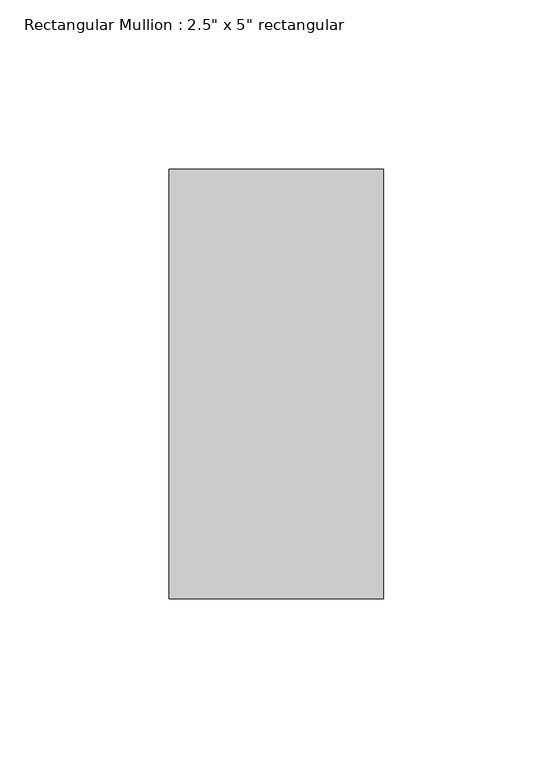
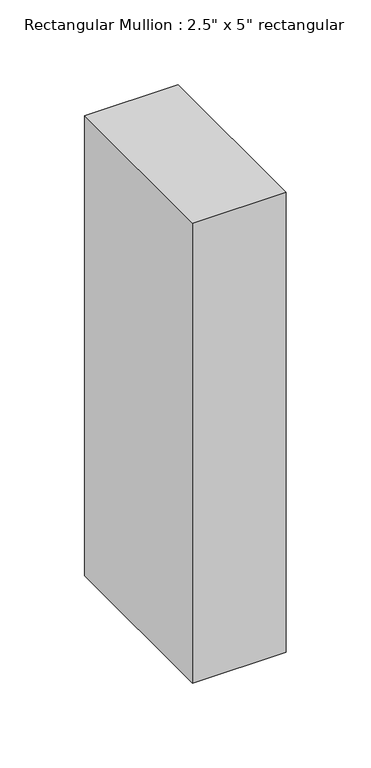
"""IFC4 building model written with IfcOpenShell, lengths in millimetres: member geometry."""

from ifc_helpers import new_model, si_unit, frame, origin, place, context, project, spatial, polyline, outline, extrude, source, transform, mapped, element, save


def member_ff9f2d30(model_context):
    return source(origin(), model_context, "Body", "SweptSolid", [
        extrude(outline(polyline([(0.0, 63.5), (0.0, -63.5), (-63.5, -63.5), (-63.5, 63.5), (0.0, 63.5)])), frame((0.0, 0.0, -330.2), z_axis=(0.0, 0.0, 1.0), x_axis=(1.0, 0.0, 0.0)), (0.0, 0.0, 1.0), 330.2),
    ])


if __name__ == "__main__":
    model = new_model("IFC4")
    model_context = context("Model", 3, world=origin())
    ifc_project = project(units=[si_unit("LENGTHUNIT", "METRE", prefix="MILLI")], contexts=[model_context])
    site = spatial("IfcSite", under=ifc_project)
    building = spatial("IfcBuilding", under=site)
    placement = place(None, origin())
    member_shape = member_ff9f2d30(model_context)
    element("IfcMember", 1, ObjectType="Rectangular Mullion : 2.5\" x 5\" rectangular", at=placement, inside=building, context=model_context, shape_type="MappedRepresentation", body=[
        mapped(member_shape, transform((0.0, 0.0, 0.0), x_axis=(1.0, 0.0, 0.0), y_axis=(0.0, 1.0, 0.0), z_axis=(0.0, 0.0, 1.0))),
    ])
    save(model, "model.ifc")

# Revit data of these elements
# Type "Rectangular Mullion : 2.5\" x 5\" rectangular"
#   built-in parameter 1007304 = 0.416667 (stored number, unit not read)
#   built-in parameter 1007301 = 0.104167 (stored number, unit not read)
#   built-in parameter 1007300 = 0.104167 (stored number, unit not read)
# Element 1 (IfcMember, "Rectangular Mullion : 2.5\" x 5\" rectangular")
#   Materials on its faces: "Aluminum"
# Materials
#   "Aluminum": class "Metal", colour RGB 247 247 247, transparency 0, Description = "Aluminum 6061", Cost = 0
